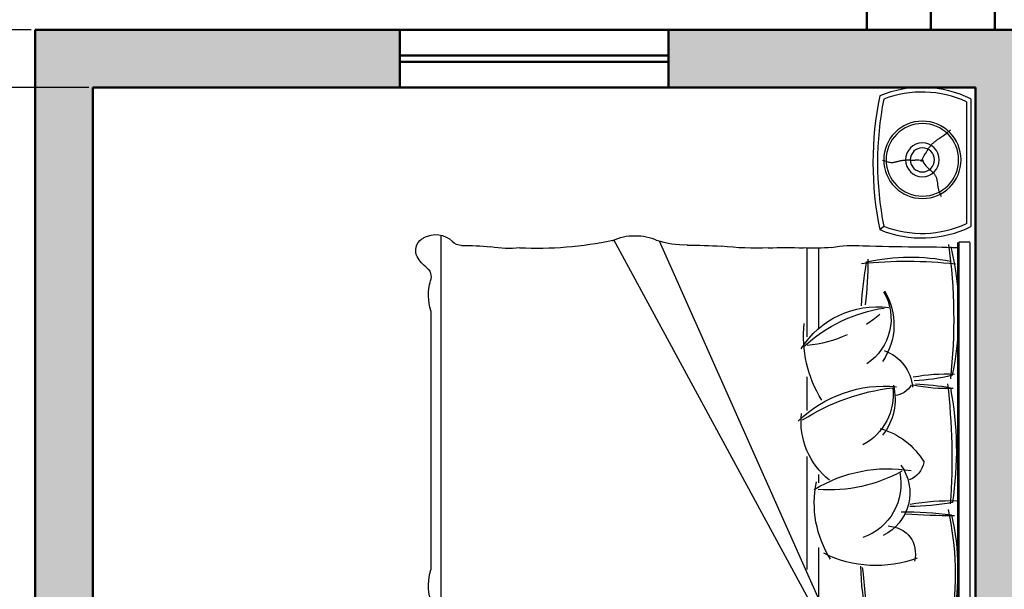
# Model space of a CAD drawing. Units: inches. Extents: x 1986 to 21484, y -1816 to 2016.
# Tile 9 of 85: x 2076 to 2230, y 1765 to 1854. Entities that reach past the tile are written whole.
import ezdxf

# ---------------------------------------------------------------- set-up
doc = ezdxf.new("R2010")
doc.units = ezdxf.units.IN
for name, color, linetype, lineweight in [('A-ANNO-DIMS', 2, 'Continuous', 18), ('A-FURN', 8, 'Continuous', 18), ('A-WALL', 7, 'Continuous', 50), ('A-WALL-PATT', 8, 'Continuous', 13)]:
    doc.layers.add(name, color=color, linetype=linetype, lineweight=lineweight)
doc.layers.add('TEFRİŞ', color=11, linetype='Continuous')
doc.styles.get("Standard").update_dxf_attribs({"font": 'arial.ttf'})
doc.dimstyles.new('ISO-25', dxfattribs={"dimtxt": 8, "dimasz": 2.5, "dimexe": 1.25, "dimexo": 0.625, "dimtad": 1, "dimdec": 1, "dimlunit": 3, "dimtxsty": 'Standard', "dimcen": 2.5, "dimadec": 0, "dimazin": 0, "dimtfac": 1, "dimtdec": 1, "dimtmove": 0, "dimatfit": 3, "dimfxl": 1, "dimarcsym": 0})

# ---------------------------------------------------------------- blocks, each defined once
blk = doc.blocks.new('BED')
at = {"layer": 'TEFRİŞ'}
for p, q in [((2114.88, 1835.66), (2129.12, 1835.66)), ((2177.29, 1835.98), (2177.61, 1835.47)), ((2177.29, 1835.98), (2191.52, 1835.98)), ((2191.2, 1835.47), (2191.52, 1835.98)), ((2115.2, 1835.15), (2128.8, 1835.15)), ((2130.81, 1834.34), (2130.81, 1835.55)), ((2130.91, 1835.55), (2175.56, 1835.55)), ((2175.56, 1835.55), (2175.56, 1834.34)), ((2177.61, 1835.47), (2191.2, 1835.47)), ((2118.49, 1833.2), (2118.34, 1833.38)), ((2118.49, 1833.2), (2118.34, 1833.38)), ((2175.56, 1834.34), (2130.81, 1834.34)), ((2175, 1834.19), (2130.91, 1834.19)), ((2180.9, 1833.52), (2180.75, 1833.7)), ((2180.9, 1833.52), (2180.75, 1833.7)), ((2181.04, 1833.35), (2180.9, 1833.52)), ((2181.04, 1833.35), (2180.9, 1833.52)), ((2118.63, 1833.03), (2118.49, 1833.2)), ((2118.63, 1833.03), (2118.49, 1833.2)), ((2118.75, 1832.88), (2118.63, 1833.03)), ((2118.75, 1832.88), (2118.63, 1833.03)), ((2118.86, 1832.74), (2118.75, 1832.88)), ((2118.86, 1832.74), (2118.75, 1832.88)), ((2118.95, 1832.61), (2118.86, 1832.74)), ((2118.95, 1832.61), (2118.86, 1832.74)), ((2119.04, 1832.48), (2118.95, 1832.61)), ((2119.04, 1832.48), (2118.95, 1832.61)), ((2119.12, 1832.37), (2119.04, 1832.48)), ((2119.12, 1832.37), (2119.04, 1832.48)), ((2119.19, 1832.26), (2119.12, 1832.37)), ((2119.19, 1832.26), (2119.12, 1832.37)), ((2125.6, 1832.25), (2125.68, 1832.3)), ((2125.6, 1832.25), (2125.68, 1832.3)), ((2125.68, 1832.3), (2125.75, 1832.35)), ((2125.68, 1832.3), (2125.75, 1832.35)), ((2181.16, 1833.2), (2181.04, 1833.35)), ((2181.16, 1833.2), (2181.04, 1833.35)), ((2181.26, 1833.06), (2181.16, 1833.2)), ((2181.26, 1833.06), (2181.16, 1833.2)), ((2181.36, 1832.93), (2181.26, 1833.06)), ((2181.36, 1832.93), (2181.26, 1833.06)), ((2181.44, 1832.8), (2181.36, 1832.93)), ((2181.44, 1832.8), (2181.36, 1832.93)), ((2181.52, 1832.69), (2181.44, 1832.8)), ((2181.52, 1832.69), (2181.44, 1832.8)), ((2181.59, 1832.58), (2181.52, 1832.69)), ((2181.59, 1832.58), (2181.52, 1832.69)), ((2181.66, 1832.48), (2181.59, 1832.58)), ((2181.66, 1832.48), (2181.59, 1832.58)), ((2181.73, 1832.38), (2181.66, 1832.48)), ((2181.73, 1832.38), (2181.66, 1832.48)), ((2181.79, 1832.29), (2181.73, 1832.38)), ((2181.79, 1832.29), (2181.73, 1832.38)), ((2181.85, 1832.21), (2181.79, 1832.29)), ((2181.85, 1832.21), (2181.79, 1832.29)), ((2186.9, 1832.26), (2186.97, 1832.27)), ((2186.9, 1832.26), (2186.97, 1832.27)), ((2186.97, 1832.27), (2187.04, 1832.28)), ((2186.97, 1832.27), (2187.04, 1832.28)), ((2187.04, 1832.28), (2187.12, 1832.3)), ((2187.04, 1832.28), (2187.12, 1832.3)), ((2187.12, 1832.3), (2187.2, 1832.31)), ((2187.12, 1832.3), (2187.2, 1832.31)), ((2187.2, 1832.31), (2187.28, 1832.33)), ((2187.2, 1832.31), (2187.28, 1832.33)), ((2187.28, 1832.33), (2187.36, 1832.35)), ((2187.28, 1832.33), (2187.36, 1832.35)), ((2187.36, 1832.35), (2187.45, 1832.37)), ((2187.36, 1832.35), (2187.45, 1832.37)), ((2187.45, 1832.37), (2187.54, 1832.4)), ((2187.45, 1832.37), (2187.54, 1832.4)), ((2187.54, 1832.4), (2187.64, 1832.43)), ((2187.54, 1832.4), (2187.64, 1832.43)), ((2187.64, 1832.43), (2187.74, 1832.46)), ((2187.64, 1832.43), (2187.74, 1832.46)), ((2187.74, 1832.46), (2187.83, 1832.49)), ((2187.74, 1832.46), (2187.83, 1832.49)), ((2187.83, 1832.49), (2187.92, 1832.53)), ((2187.83, 1832.49), (2187.92, 1832.53)), ((2187.92, 1832.53), (2188.01, 1832.57)), ((2187.92, 1832.53), (2188.01, 1832.57)), ((2188.01, 1832.57), (2188.09, 1832.62)), ((2188.01, 1832.57), (2188.09, 1832.62)), ((2188.09, 1832.62), (2188.15, 1832.67)), ((2188.09, 1832.62), (2188.15, 1832.67)), ((2119.26, 1832.16), (2119.19, 1832.26)), ((2119.26, 1832.16), (2119.19, 1832.26)), ((2119.32, 1832.06), (2119.26, 1832.16)), ((2119.32, 1832.06), (2119.26, 1832.16)), ((2119.39, 1831.97), (2119.32, 1832.06)), ((2119.39, 1831.97), (2119.32, 1832.06)), ((2119.45, 1831.89), (2119.39, 1831.97)), ((2119.45, 1831.89), (2119.39, 1831.97)), ((2119.51, 1831.81), (2119.45, 1831.89)), ((2119.51, 1831.81), (2119.45, 1831.89)), ((2119.57, 1831.73), (2119.51, 1831.81)), ((2119.57, 1831.73), (2119.51, 1831.81)), ((2119.63, 1831.65), (2119.57, 1831.73)), ((2119.63, 1831.65), (2119.57, 1831.73)), ((2119.69, 1831.58), (2119.63, 1831.65)), ((2119.69, 1831.58), (2119.63, 1831.65)), ((2119.75, 1831.51), (2119.69, 1831.58)), ((2119.75, 1831.51), (2119.69, 1831.58)), ((2119.81, 1831.44), (2119.75, 1831.51)), ((2119.81, 1831.44), (2119.75, 1831.51)), ((2119.87, 1831.38), (2119.81, 1831.44)), ((2119.87, 1831.38), (2119.81, 1831.44)), ((2119.93, 1831.31), (2119.87, 1831.38)), ((2119.93, 1831.31), (2119.87, 1831.38)), ((2119.99, 1831.25), (2119.93, 1831.31)), ((2119.99, 1831.25), (2119.93, 1831.31)), ((2120.05, 1831.2), (2119.99, 1831.25)), ((2120.05, 1831.2), (2119.99, 1831.25)), ((2120.12, 1831.14), (2120.05, 1831.2)), ((2120.12, 1831.14), (2120.05, 1831.2)), ((2122.8, 1831.09), (2122.87, 1831.18)), ((2122.8, 1831.09), (2122.87, 1831.18)), ((2122.87, 1831.18), (2122.94, 1831.26)), ((2122.87, 1831.18), (2122.94, 1831.26)), ((2122.94, 1831.26), (2123.01, 1831.33)), ((2122.94, 1831.26), (2123.01, 1831.33)), ((2123.01, 1831.33), (2123.08, 1831.4)), ((2123.01, 1831.33), (2123.08, 1831.4)), ((2123.08, 1831.4), (2123.14, 1831.46)), ((2123.08, 1831.4), (2123.14, 1831.46)), ((2123.14, 1831.46), (2123.21, 1831.52)), ((2123.14, 1831.46), (2123.21, 1831.52)), ((2123.21, 1831.52), (2123.27, 1831.58)), ((2123.21, 1831.52), (2123.27, 1831.58)), ((2123.27, 1831.58), (2123.34, 1831.63)), ((2123.27, 1831.58), (2123.34, 1831.63)), ((2123.34, 1831.63), (2123.41, 1831.67)), ((2123.34, 1831.63), (2123.41, 1831.67)), ((2123.41, 1831.67), (2123.48, 1831.71)), ((2123.41, 1831.67), (2123.48, 1831.71)), ((2123.48, 1831.71), (2123.55, 1831.74)), ((2123.48, 1831.71), (2123.55, 1831.74)), ((2123.55, 1831.74), (2123.62, 1831.77)), ((2123.55, 1831.74), (2123.62, 1831.77)), ((2123.62, 1831.77), (2123.69, 1831.8)), ((2123.62, 1831.77), (2123.69, 1831.8)), ((2123.69, 1831.8), (2123.77, 1831.82)), ((2123.69, 1831.8), (2123.77, 1831.82)), ((2123.77, 1831.82), (2123.84, 1831.84)), ((2123.77, 1831.82), (2123.84, 1831.84)), ((2123.84, 1831.84), (2123.91, 1831.86)), ((2123.84, 1831.84), (2123.91, 1831.86)), ((2123.91, 1831.86), (2123.98, 1831.87)), ((2123.91, 1831.86), (2123.98, 1831.87)), ((2123.98, 1831.87), (2124.06, 1831.89)), ((2123.98, 1831.87), (2124.06, 1831.89)), ((2124.06, 1831.89), (2124.13, 1831.9)), ((2124.06, 1831.89), (2124.13, 1831.9)), ((2124.13, 1831.9), (2124.2, 1831.91)), ((2124.13, 1831.9), (2124.2, 1831.91)), ((2124.2, 1831.91), (2124.27, 1831.91)), ((2124.2, 1831.91), (2124.27, 1831.91)), ((2124.27, 1831.91), (2124.35, 1831.92)), ((2124.27, 1831.91), (2124.35, 1831.92)), ((2124.35, 1831.92), (2124.42, 1831.93)), ((2124.35, 1831.92), (2124.42, 1831.93)), ((2124.42, 1831.93), (2124.49, 1831.94)), ((2124.42, 1831.93), (2124.49, 1831.94)), ((2124.49, 1831.94), (2124.56, 1831.95)), ((2124.49, 1831.94), (2124.56, 1831.95)), ((2124.56, 1831.95), (2124.64, 1831.96)), ((2124.56, 1831.95), (2124.64, 1831.96)), ((2124.64, 1831.96), (2124.71, 1831.98)), ((2124.64, 1831.96), (2124.71, 1831.98)), ((2124.71, 1831.98), (2124.79, 1831.99)), ((2124.71, 1831.98), (2124.79, 1831.99)), ((2124.79, 1831.99), (2124.87, 1832.01)), ((2124.79, 1831.99), (2124.87, 1832.01)), ((2124.87, 1832.01), (2124.96, 1832.03)), ((2124.87, 1832.01), (2124.96, 1832.03)), ((2124.96, 1832.03), (2125.05, 1832.05)), ((2124.96, 1832.03), (2125.05, 1832.05)), ((2125.05, 1832.05), (2125.14, 1832.08)), ((2125.05, 1832.05), (2125.14, 1832.08)), ((2125.14, 1832.08), (2125.23, 1832.11)), ((2125.14, 1832.08), (2125.23, 1832.11)), ((2125.23, 1832.11), (2125.33, 1832.14)), ((2125.23, 1832.11), (2125.33, 1832.14)), ((2125.33, 1832.14), (2125.42, 1832.17)), ((2125.33, 1832.14), (2125.42, 1832.17)), ((2125.42, 1832.17), (2125.52, 1832.21)), ((2125.42, 1832.17), (2125.52, 1832.21)), ((2125.52, 1832.21), (2125.6, 1832.25)), ((2125.52, 1832.21), (2125.6, 1832.25)), ((2181.92, 1832.13), (2181.85, 1832.21)), ((2181.92, 1832.13), (2181.85, 1832.21)), ((2181.97, 1832.05), (2181.92, 1832.13)), ((2181.97, 1832.05), (2181.92, 1832.13)), ((2182.03, 1831.97), (2181.97, 1832.05)), ((2182.03, 1831.97), (2181.97, 1832.05)), ((2182.09, 1831.9), (2182.03, 1831.97)), ((2182.09, 1831.9), (2182.03, 1831.97)), ((2182.15, 1831.83), (2182.09, 1831.9)), ((2182.15, 1831.83), (2182.09, 1831.9)), ((2182.21, 1831.76), (2182.15, 1831.83)), ((2182.21, 1831.76), (2182.15, 1831.83)), ((2182.27, 1831.7), (2182.21, 1831.76)), ((2182.27, 1831.7), (2182.21, 1831.76)), ((2182.33, 1831.63), (2182.27, 1831.7)), ((2182.33, 1831.63), (2182.27, 1831.7)), ((2182.4, 1831.57), (2182.33, 1831.63)), ((2182.4, 1831.57), (2182.33, 1831.63)), ((2182.46, 1831.52), (2182.4, 1831.57)), ((2182.46, 1831.52), (2182.4, 1831.57)), ((2182.52, 1831.46), (2182.46, 1831.52)), ((2182.52, 1831.46), (2182.46, 1831.52)), ((2182.59, 1831.41), (2182.52, 1831.46)), ((2182.59, 1831.41), (2182.52, 1831.46)), ((2182.66, 1831.36), (2182.59, 1831.41)), ((2182.66, 1831.36), (2182.59, 1831.41)), ((2182.73, 1831.31), (2182.66, 1831.36)), ((2182.73, 1831.31), (2182.66, 1831.36)), ((2182.8, 1831.26), (2182.73, 1831.31)), ((2182.8, 1831.26), (2182.73, 1831.31)), ((2182.87, 1831.22), (2182.8, 1831.26)), ((2182.87, 1831.22), (2182.8, 1831.26)), ((2182.95, 1831.17), (2182.87, 1831.22)), ((2182.95, 1831.17), (2182.87, 1831.22)), ((2183.03, 1831.12), (2182.95, 1831.17)), ((2183.03, 1831.12), (2182.95, 1831.17)), ((2184.95, 1831.14), (2185.05, 1831.23)), ((2184.95, 1831.14), (2185.05, 1831.23)), ((2185.05, 1831.23), (2185.13, 1831.33)), ((2185.05, 1831.23), (2185.13, 1831.33)), ((2185.13, 1831.33), (2185.21, 1831.41)), ((2185.13, 1831.33), (2185.21, 1831.41)), ((2185.21, 1831.41), (2185.28, 1831.5)), ((2185.21, 1831.41), (2185.28, 1831.5)), ((2185.28, 1831.5), (2185.35, 1831.58)), ((2185.28, 1831.5), (2185.35, 1831.58)), ((2185.35, 1831.58), (2185.42, 1831.65)), ((2185.35, 1831.58), (2185.42, 1831.65)), ((2185.42, 1831.65), (2185.48, 1831.72)), ((2185.42, 1831.65), (2185.48, 1831.72)), ((2185.48, 1831.72), (2185.55, 1831.78)), ((2185.48, 1831.72), (2185.55, 1831.78)), ((2185.55, 1831.78), (2185.61, 1831.84)), ((2185.55, 1831.78), (2185.61, 1831.84)), ((2185.61, 1831.84), (2185.68, 1831.9)), ((2185.61, 1831.84), (2185.68, 1831.9)), ((2185.68, 1831.9), (2185.75, 1831.95)), ((2185.68, 1831.9), (2185.75, 1831.95)), ((2185.75, 1831.95), (2185.82, 1831.99)), ((2185.75, 1831.95), (2185.82, 1831.99)), ((2185.82, 1831.99), (2185.89, 1832.03)), ((2185.82, 1831.99), (2185.89, 1832.03)), ((2185.89, 1832.03), (2185.96, 1832.06)), ((2185.89, 1832.03), (2185.96, 1832.06)), ((2185.96, 1832.06), (2186.03, 1832.09)), ((2185.96, 1832.06), (2186.03, 1832.09)), ((2186.03, 1832.09), (2186.1, 1832.12)), ((2186.03, 1832.09), (2186.1, 1832.12)), ((2186.1, 1832.12), (2186.17, 1832.14)), ((2186.1, 1832.12), (2186.17, 1832.14)), ((2186.17, 1832.14), (2186.24, 1832.16)), ((2186.17, 1832.14), (2186.24, 1832.16)), ((2186.24, 1832.16), (2186.32, 1832.18)), ((2186.24, 1832.16), (2186.32, 1832.18)), ((2186.32, 1832.18), (2186.39, 1832.19)), ((2186.32, 1832.18), (2186.39, 1832.19)), ((2186.39, 1832.19), (2186.46, 1832.21)), ((2186.39, 1832.19), (2186.46, 1832.21)), ((2186.46, 1832.21), (2186.53, 1832.22)), ((2186.46, 1832.21), (2186.53, 1832.22)), ((2186.53, 1832.22), (2186.61, 1832.23)), ((2186.53, 1832.22), (2186.61, 1832.23)), ((2186.61, 1832.23), (2186.68, 1832.23)), ((2186.61, 1832.23), (2186.68, 1832.23)), ((2186.68, 1832.23), (2186.75, 1832.24)), ((2186.68, 1832.23), (2186.75, 1832.24)), ((2186.75, 1832.24), (2186.82, 1832.25)), ((2186.75, 1832.24), (2186.82, 1832.25)), ((2186.82, 1832.25), (2186.9, 1832.26)), ((2186.82, 1832.25), (2186.9, 1832.26)), ((2120.18, 1831.09), (2120.12, 1831.14)), ((2120.18, 1831.09), (2120.12, 1831.14)), ((2120.25, 1831.04), (2120.18, 1831.09)), ((2120.25, 1831.04), (2120.18, 1831.09)), ((2120.32, 1830.99), (2120.25, 1831.04)), ((2120.32, 1830.99), (2120.25, 1831.04)), ((2120.39, 1830.94), (2120.32, 1830.99)), ((2120.39, 1830.94), (2120.32, 1830.99)), ((2120.47, 1830.9), (2120.39, 1830.94)), ((2120.47, 1830.9), (2120.39, 1830.94)), ((2120.54, 1830.85), (2120.47, 1830.9)), ((2120.54, 1830.85), (2120.47, 1830.9)), ((2120.62, 1830.8), (2120.54, 1830.85)), ((2120.62, 1830.8), (2120.54, 1830.85)), ((2120.7, 1830.75), (2120.62, 1830.8)), ((2120.7, 1830.75), (2120.62, 1830.8)), ((2120.79, 1830.7), (2120.7, 1830.75)), ((2120.79, 1830.7), (2120.7, 1830.75)), ((2120.88, 1830.65), (2120.79, 1830.7)), ((2120.88, 1830.65), (2120.79, 1830.7)), ((2120.98, 1830.59), (2120.88, 1830.65)), ((2120.98, 1830.59), (2120.88, 1830.65)), ((2121.09, 1830.52), (2120.98, 1830.59)), ((2121.09, 1830.52), (2120.98, 1830.59)), ((2121.21, 1830.45), (2121.09, 1830.52)), ((2121.21, 1830.45), (2121.09, 1830.52)), ((2121.34, 1830.38), (2121.21, 1830.45)), ((2121.34, 1830.38), (2121.21, 1830.45)), ((2121.49, 1830.29), (2121.34, 1830.38)), ((2121.49, 1830.29), (2121.34, 1830.38)), ((2121.66, 1830.21), (2121.49, 1830.29)), ((2121.66, 1830.21), (2121.49, 1830.29)), ((2121.66, 1830.18), (2121.87, 1830.29)), ((2121.66, 1830.18), (2121.87, 1830.29)), ((2121.85, 1830.11), (2121.66, 1830.21)), ((2121.85, 1830.11), (2121.66, 1830.21)), ((2121.76, 1830.38), (2121.74, 1830.17)), ((2121.76, 1830.38), (2121.74, 1830.17)), ((2121.74, 1830.17), (2121.74, 1829.99)), ((2121.74, 1830.17), (2121.74, 1829.99)), ((2121.87, 1830.29), (2122.04, 1830.4)), ((2121.87, 1830.29), (2122.04, 1830.4)), ((2122.04, 1830.4), (2122.2, 1830.51)), ((2122.04, 1830.4), (2122.2, 1830.51)), ((2122.2, 1830.51), (2122.33, 1830.61)), ((2122.2, 1830.51), (2122.33, 1830.61)), ((2122.33, 1830.61), (2122.45, 1830.72)), ((2122.33, 1830.61), (2122.45, 1830.72)), ((2122.45, 1830.72), (2122.55, 1830.82)), ((2122.45, 1830.72), (2122.55, 1830.82)), ((2122.55, 1830.82), (2122.64, 1830.91)), ((2122.55, 1830.82), (2122.64, 1830.91)), ((2122.64, 1830.91), (2122.72, 1831.01)), ((2122.64, 1830.91), (2122.72, 1831.01)), ((2122.72, 1831.01), (2122.8, 1831.09)), ((2122.72, 1831.01), (2122.8, 1831.09)), ((2183.11, 1831.07), (2183.03, 1831.12)), ((2183.11, 1831.07), (2183.03, 1831.12)), ((2183.2, 1831.02), (2183.11, 1831.07)), ((2183.2, 1831.02), (2183.11, 1831.07)), ((2183.29, 1830.97), (2183.2, 1831.02)), ((2183.29, 1830.97), (2183.2, 1831.02)), ((2183.39, 1830.91), (2183.29, 1830.97)), ((2183.39, 1830.91), (2183.29, 1830.97)), ((2183.49, 1830.84), (2183.39, 1830.91)), ((2183.49, 1830.84), (2183.39, 1830.91)), ((2183.61, 1830.77), (2183.49, 1830.84)), ((2183.61, 1830.77), (2183.49, 1830.84)), ((2183.75, 1830.7), (2183.61, 1830.77)), ((2183.75, 1830.7), (2183.61, 1830.77)), ((2183.9, 1830.61), (2183.75, 1830.7)), ((2183.9, 1830.61), (2183.75, 1830.7)), ((2184.06, 1830.53), (2183.9, 1830.61)), ((2184.06, 1830.53), (2183.9, 1830.61)), ((2184.25, 1830.43), (2184.06, 1830.53)), ((2184.25, 1830.43), (2184.06, 1830.53)), ((2184.07, 1830.5), (2184.27, 1830.61)), ((2184.07, 1830.5), (2184.27, 1830.61)), ((2184.15, 1830.49), (2184.14, 1830.31)), ((2184.15, 1830.49), (2184.14, 1830.31)), ((2184.14, 1830.31), (2184.14, 1830.15)), ((2184.14, 1830.31), (2184.14, 1830.15)), ((2184.14, 1830.15), (2184.14, 1830.01)), ((2184.14, 1830.15), (2184.14, 1830.01)), ((2184.17, 1830.7), (2184.15, 1830.49)), ((2184.17, 1830.7), (2184.15, 1830.49)), ((2184.27, 1830.61), (2184.45, 1830.72)), ((2184.27, 1830.61), (2184.45, 1830.72)), ((2184.45, 1830.72), (2184.6, 1830.83)), ((2184.45, 1830.72), (2184.6, 1830.83)), ((2184.6, 1830.83), (2184.74, 1830.93)), ((2184.6, 1830.83), (2184.74, 1830.93)), ((2184.74, 1830.93), (2184.85, 1831.04)), ((2184.74, 1830.93), (2184.85, 1831.04)), ((2184.85, 1831.04), (2184.95, 1831.14)), ((2184.85, 1831.04), (2184.95, 1831.14)), ((2121.74, 1829.99), (2121.73, 1829.83)), ((2121.74, 1829.99), (2121.73, 1829.83)), ((2121.73, 1829.83), (2121.73, 1829.69)), ((2121.73, 1829.83), (2121.73, 1829.69)), ((2121.73, 1829.69), (2121.73, 1829.57)), ((2121.73, 1829.69), (2121.73, 1829.57)), ((2121.73, 1829.57), (2121.73, 1829.45)), ((2121.73, 1829.57), (2121.73, 1829.45)), ((2121.73, 1829.45), (2121.74, 1829.35)), ((2121.73, 1829.45), (2121.74, 1829.35)), ((2121.74, 1829.35), (2121.74, 1829.25)), ((2121.74, 1829.35), (2121.74, 1829.25)), ((2121.74, 1829.25), (2121.74, 1829.16)), ((2121.74, 1829.25), (2121.74, 1829.16)), ((2121.74, 1829.16), (2121.74, 1829.06)), ((2121.74, 1829.16), (2121.74, 1829.06)), ((2121.74, 1829.06), (2121.74, 1828.97)), ((2121.74, 1829.06), (2121.74, 1828.97)), ((2121.74, 1828.97), (2121.74, 1828.89)), ((2121.74, 1828.97), (2121.74, 1828.89)), ((2184.14, 1829.04), (2184.13, 1828.96)), ((2184.14, 1829.04), (2184.13, 1828.96)), ((2184.14, 1830.01), (2184.14, 1829.89)), ((2184.14, 1830.01), (2184.14, 1829.89)), ((2184.14, 1829.89), (2184.14, 1829.77)), ((2184.14, 1829.89), (2184.14, 1829.77)), ((2184.14, 1829.77), (2184.14, 1829.67)), ((2184.14, 1829.77), (2184.14, 1829.67)), ((2184.14, 1829.67), (2184.15, 1829.57)), ((2184.14, 1829.67), (2184.15, 1829.57)), ((2184.15, 1829.38), (2184.14, 1829.29)), ((2184.15, 1829.38), (2184.14, 1829.29)), ((2184.14, 1829.29), (2184.14, 1829.21)), ((2184.14, 1829.29), (2184.14, 1829.21)), ((2184.14, 1829.21), (2184.14, 1829.12)), ((2184.14, 1829.21), (2184.14, 1829.12)), ((2184.14, 1829.12), (2184.14, 1829.04)), ((2184.14, 1829.12), (2184.14, 1829.04)), ((2184.15, 1829.57), (2184.15, 1829.48)), ((2184.15, 1829.57), (2184.15, 1829.48)), ((2184.15, 1829.48), (2184.15, 1829.38)), ((2184.15, 1829.48), (2184.15, 1829.38)), ((2121.74, 1828.89), (2121.73, 1828.8)), ((2121.74, 1828.89), (2121.73, 1828.8)), ((2121.73, 1828.8), (2121.73, 1828.72)), ((2121.73, 1828.8), (2121.73, 1828.72)), ((2121.73, 1828.72), (2121.73, 1828.64)), ((2121.73, 1828.72), (2121.73, 1828.64)), ((2121.73, 1828.64), (2121.73, 1828.56)), ((2121.73, 1828.64), (2121.73, 1828.56)), ((2121.73, 1828.56), (2121.73, 1828.48)), ((2121.73, 1828.56), (2121.73, 1828.48)), ((2121.73, 1828.48), (2121.73, 1828.4)), ((2121.73, 1828.48), (2121.73, 1828.4)), ((2121.73, 1828.4), (2121.73, 1828.33)), ((2121.73, 1828.4), (2121.73, 1828.33)), ((2121.73, 1828.33), (2121.74, 1828.25)), ((2121.73, 1828.33), (2121.74, 1828.25)), ((2121.74, 1828.25), (2121.75, 1828.18)), ((2121.74, 1828.25), (2121.75, 1828.18)), ((2121.75, 1828.18), (2121.75, 1828.1)), ((2121.75, 1828.18), (2121.75, 1828.1)), ((2121.75, 1828.1), (2121.76, 1828.03)), ((2121.75, 1828.1), (2121.76, 1828.03)), ((2121.76, 1828.03), (2121.78, 1827.95)), ((2121.76, 1828.03), (2121.78, 1827.95)), ((2121.78, 1827.95), (2121.79, 1827.88)), ((2121.78, 1827.95), (2121.79, 1827.88)), ((2121.79, 1827.88), (2121.8, 1827.8)), ((2121.79, 1827.88), (2121.8, 1827.8)), ((2184.13, 1828.96), (2184.13, 1828.88)), ((2184.13, 1828.96), (2184.13, 1828.88)), ((2184.13, 1828.88), (2184.13, 1828.8)), ((2184.13, 1828.88), (2184.13, 1828.8)), ((2184.13, 1828.8), (2184.14, 1828.72)), ((2184.13, 1828.8), (2184.14, 1828.72)), ((2184.14, 1828.72), (2184.14, 1828.65)), ((2184.14, 1828.72), (2184.14, 1828.65)), ((2184.14, 1828.65), (2184.15, 1828.57)), ((2184.14, 1828.65), (2184.15, 1828.57)), ((2184.15, 1828.57), (2184.15, 1828.5)), ((2184.15, 1828.57), (2184.15, 1828.5)), ((2184.15, 1828.5), (2184.16, 1828.42)), ((2184.15, 1828.5), (2184.16, 1828.42)), ((2184.16, 1828.42), (2184.17, 1828.35)), ((2184.16, 1828.42), (2184.17, 1828.35)), ((2184.17, 1828.35), (2184.18, 1828.27)), ((2184.17, 1828.35), (2184.18, 1828.27)), ((2184.18, 1828.27), (2184.19, 1828.2)), ((2184.18, 1828.27), (2184.19, 1828.2)), ((2184.19, 1828.2), (2184.21, 1828.12)), ((2184.19, 1828.2), (2184.21, 1828.12)), ((2184.21, 1828.12), (2184.22, 1828.04)), ((2184.21, 1828.12), (2184.22, 1828.04)), ((2184.22, 1828.04), (2184.24, 1827.97)), ((2184.22, 1828.04), (2184.24, 1827.97)), ((2184.24, 1827.97), (2184.26, 1827.89)), ((2184.24, 1827.97), (2184.26, 1827.89)), ((2184.26, 1827.89), (2184.28, 1827.81)), ((2184.26, 1827.89), (2184.28, 1827.81)), ((2121.8, 1827.8), (2121.82, 1827.72)), ((2121.8, 1827.8), (2121.82, 1827.72)), ((2121.82, 1827.72), (2121.84, 1827.65)), ((2121.82, 1827.72), (2121.84, 1827.65)), ((2121.84, 1827.65), (2121.85, 1827.57)), ((2121.84, 1827.65), (2121.85, 1827.57)), ((2121.85, 1827.57), (2121.87, 1827.49)), ((2121.85, 1827.57), (2121.87, 1827.49)), ((2121.87, 1827.49), (2121.89, 1827.41)), ((2121.87, 1827.49), (2121.89, 1827.41)), ((2121.89, 1827.41), (2121.91, 1827.33)), ((2121.89, 1827.41), (2121.91, 1827.33)), ((2121.91, 1827.33), (2121.93, 1827.26)), ((2121.91, 1827.33), (2121.93, 1827.26)), ((2121.93, 1827.26), (2121.95, 1827.18)), ((2121.93, 1827.26), (2121.95, 1827.18)), ((2121.95, 1827.18), (2121.97, 1827.09)), ((2121.95, 1827.18), (2121.97, 1827.09)), ((2121.97, 1827.09), (2121.99, 1827.01)), ((2121.97, 1827.09), (2121.99, 1827.01)), ((2121.99, 1827.01), (2122, 1826.93)), ((2121.99, 1827.01), (2122, 1826.93)), ((2122, 1826.93), (2122.01, 1826.84)), ((2122, 1826.93), (2122.01, 1826.84)), ((2122.01, 1826.84), (2122, 1826.74)), ((2122.01, 1826.84), (2122, 1826.74)), ((2184.28, 1827.81), (2184.3, 1827.73)), ((2184.28, 1827.81), (2184.3, 1827.73)), ((2184.3, 1827.73), (2184.32, 1827.65)), ((2184.3, 1827.73), (2184.32, 1827.65)), ((2184.32, 1827.65), (2184.34, 1827.58)), ((2184.32, 1827.65), (2184.34, 1827.58)), ((2184.34, 1827.58), (2184.36, 1827.5)), ((2184.34, 1827.58), (2184.36, 1827.5)), ((2184.38, 1826.86), (2184.35, 1826.74)), ((2184.38, 1826.86), (2184.35, 1826.74)), ((2184.36, 1827.5), (2184.38, 1827.41)), ((2184.36, 1827.5), (2184.38, 1827.41)), ((2184.38, 1827.41), (2184.4, 1827.33)), ((2184.38, 1827.41), (2184.4, 1827.33)), ((2184.4, 1826.96), (2184.38, 1826.86)), ((2184.4, 1826.96), (2184.38, 1826.86)), ((2184.4, 1827.33), (2184.41, 1827.25)), ((2184.4, 1827.33), (2184.41, 1827.25)), ((2184.41, 1827.06), (2184.4, 1826.96)), ((2184.41, 1827.06), (2184.4, 1826.96)), ((2184.41, 1827.25), (2184.41, 1827.16)), ((2184.41, 1827.25), (2184.41, 1827.16)), ((2184.41, 1827.16), (2184.41, 1827.06)), ((2184.41, 1827.16), (2184.41, 1827.06)), ((2121.78, 1825.93), (2121.74, 1825.8)), ((2121.78, 1825.93), (2121.74, 1825.8)), ((2121.83, 1826.06), (2121.78, 1825.93)), ((2121.83, 1826.06), (2121.78, 1825.93)), ((2121.87, 1826.19), (2121.83, 1826.06)), ((2121.87, 1826.19), (2121.83, 1826.06)), ((2121.91, 1826.31), (2121.87, 1826.19)), ((2121.91, 1826.31), (2121.87, 1826.19)), ((2121.95, 1826.42), (2121.91, 1826.31)), ((2121.95, 1826.42), (2121.91, 1826.31)), ((2121.97, 1826.54), (2121.95, 1826.42)), ((2121.97, 1826.54), (2121.95, 1826.42)), ((2121.99, 1826.64), (2121.97, 1826.54)), ((2121.99, 1826.64), (2121.97, 1826.54)), ((2122, 1826.74), (2121.99, 1826.64)), ((2122, 1826.74), (2121.99, 1826.64)), ((2129.46, 1825.49), (2129.09, 1825.93)), ((2176.94, 1825.81), (2177.31, 1826.25)), ((2184.19, 1826.25), (2184.14, 1826.12)), ((2184.19, 1826.25), (2184.14, 1826.12)), ((2184.23, 1826.38), (2184.19, 1826.25)), ((2184.23, 1826.38), (2184.19, 1826.25)), ((2184.28, 1826.51), (2184.23, 1826.38)), ((2184.28, 1826.51), (2184.23, 1826.38)), ((2184.32, 1826.63), (2184.28, 1826.51)), ((2184.32, 1826.63), (2184.28, 1826.51)), ((2184.35, 1826.74), (2184.32, 1826.63)), ((2184.35, 1826.74), (2184.32, 1826.63)), ((2191.87, 1825.81), (2191.5, 1826.25)), ((2174.77, 1820.53), (2130.76, 1800.91)), ((2174.77, 1819.77), (2130.6, 1795.83)), ((2140.43, 1818.69), (2131.53, 1818.69)), ((2157.71, 1818.69), (2156.77, 1818.69)), ((2170.41, 1818.69), (2164.92, 1818.69)), ((2141.43, 1817.4), (2131.53, 1817.4)), ((2149.62, 1817.4), (2145.88, 1817.4)), ((2167.36, 1817.4), (2154.77, 1817.4)), ((2175, 1776.57), (2130.11, 1776.57)), ((2138.52, 1775.41), (2167.39, 1775.41))]:
    blk.add_line(p, q, dxfattribs=at)
for centre, radius, start, end in [((2126, 1830.19), 12.39, 153.8162, 202.314), ((2118, 1830.19), 12.39, 337.686, 26.1838), ((2188.4, 1830.51), 12.39, 153.8162, 202.314), ((2180.41, 1830.51), 12.39, 337.686, 26.1838), ((2126, 1830.19), 11.88, 155.3335, 201.0157), ((2118, 1830.19), 11.88, 338.9843, 24.6665), ((2188.4, 1830.51), 11.88, 155.3335, 201.0157), ((2180.41, 1830.51), 11.88, 338.9843, 24.6665), ((2122, 1861.35), 36.12, 258.6773, 281.3227), ((2184.41, 1861.67), 36.63, 258.2443, 281.7557), ((2184.41, 1861.67), 36.12, 258.6773, 281.3227), ((2122, 1861.35), 36.63, 258.2443, 281.7557)]:
    blk.add_arc(centre, radius, start, end, dxfattribs=at)
at = {"layer": 'TEFRİŞ', "extrusion": (0, 0, -1)}
for centre, major_axis, ratio, start_param, end_param in [((2121.68, 1830.24), (-3.05, -3.05), 1, 3.926991, 10.210176), ((2121.68, 1830.24), (2.86, -2.86), 1, 5.497787, 11.780972), ((2121.68, 1830.24), (2.86, -2.86), 1, 5.497787, 11.780972), ((2138.85, 1803.05), (-22.1, 22.1), 1, 0.544604, 1.006234), ((2184.09, 1830.56), (-3.05, -3.05), 1, 3.926991, 10.210176), ((2184.09, 1830.56), (2.86, -2.86), 1, 5.497787, 11.780972), ((2184.09, 1830.56), (2.86, -2.86), 1, 5.497787, 11.780972), ((2139.43, 1773.84), (-42.35, 42.35), 1, 0.646251, 0.896949), ((2206.14, 1830.73), (-52.86, -52.86), 1, 0.767743, 0.83177), ((2154.7, 1828.89), (-15.68, 15.68), 1, -1.00675, -0.580436), ((2181.61, 1828.44), (-34.39, 34.39), 1, -0.888486, -0.672463), ((2164.51, 1832.79), (-13.41, 13.41), 1, -0.974476, -0.730892), ((2127.6, 1828.81), (-13.23, 13.23), 1, 2.100388, 2.328052), ((2155, 1761.9), (-50.65, -50.65), 1, 2.239512, 2.426533), ((2172.01, 1828.66), (-17.93, 17.93), 1, -0.753394, -0.598744), ((2128.44, 1832.96), (-13.26, -13.26), 1, 3.889049, 4.127298), ((2154.12, 1796.61), (-26.46, 26.46), 1, 0.596409, 0.940188), ((2183.72, 1833.22), (-17, 17), 1, -0.967105, -0.749712), ((2134, 1828.8), (-18.62, 18.62), 1, 2.173461, 2.355043), ((2168.35, 1789.27), (-1.33, 44.62), 0.875277, -0.163954, 0.163954), ((2199.2, 1828.45), (-27.06, -27.06), 1, 0.770625, 0.917228), ((2087.32, 1833.96), (-52.37, 52.37), 1, 2.358049, 2.431787), ((2167.6, 1797.72), (-0.51, 36.47), 0.865194, -0.185965, 0.185965), ((2164.15, 1828.7), (-6.99, 6.99), 1, 1.789136, 2.946702), ((2156.76, 1828.98), (-11.9, -11.9), 1, 3.646453, 4.226155), ((2099.77, 1830.73), (-52.86, 52.86), 1, 2.311571, 2.373849), ((2184.09, 1830.56), (1.33, -1.33), 1, 5.497787, 11.780972), ((2184.09, 1830.56), (1.33, -1.33), 1, 5.497787, 11.780972), ((2121.68, 1830.24), (1.33, -1.33), 1, 5.497787, 11.780972), ((2121.68, 1830.24), (1.33, -1.33), 1, 5.497787, 11.780972), ((2121.68, 1830.24), (0.952, -0.952), 1, 5.497787, 11.780972), ((2121.68, 1830.24), (0.952, -0.952), 1, 5.497787, 11.780972), ((2184.09, 1830.56), (0.952, -0.952), 1, 5.497787, 11.780972), ((2184.09, 1830.56), (0.952, -0.952), 1, 5.497787, 11.780972), ((2159.55, 1823.33), (-5.81, 5.81), 1, -0.516587, 0.256776), ((2154.84, 1827.75), (-1.93, 1.93), 1, 0.997904, 1.977819), ((2675.38, 1815.09), (-384.79, -384.79), 1, 0.80103, 0.811711), ((2147.44, 1824.41), (-3.36, -3.36), 1, 1.11934, 2.270556), ((2145.66, 1827.01), (-1.62, 1.62), 1, 1.310976, 2.284591), ((2172, 1826.44), (-11.23, 11.23), 1, -1.332486, -0.624868), ((2158.82, 1823.55), (-3.74, -3.74), 1, 1.730792, 3.47045), ((2166.67, 1824.96), (-2.93, 3.91), 0.760601, -0.723751, 0.723751), ((2153.88, 1825.05), (-9.22, 9.22), 1, 1.994956, 2.818753), ((1630.53, 1815.09), (-384.79, 384.79), 1, 2.329881, 2.340562), ((2141.71, 1819.83), (-11.86, 11.86), 1, 1.850844, 2.42862), ((2157.83, 1821.53), (-4.47, 4.47), 1, 0.576679, 2.021689), ((2140.05, 1819.86), (-5.1, 5.1), 1, 0.238357, 1.390139), ((2139.42, 1820.79), (-4.21, -4.21), 1, 1.82161, 3.349145), ((2160.6, 1825.98), (-9.68, -9.68), 1, 0.009196, 0.886853), ((2148.35, 1820.65), (-4.63, -4.63), 1, 2.117602, 3.020837), ((2147.86, 1820.64), (-4.48, 4.48), 1, 0.665914, 1.867503), ((2170.68, 1829.67), (-16.79, 16.79), 1, -1.354718, -0.902276), ((2148.15, 1825.25), (-7.14, -7.14), 1, 6.061986, 7.190757), ((2154.93, 1828.48), (-11.96, 11.96), 1, -1.530302, -0.934407), ((2127.37, 1815.76), (-10.68, 10.68), 1, 1.657204, 1.779381), ((2146.08, 1822.57), (-10.5, 10.5), 1, -0.951783, -0.716225), ((2132.43, 1774.09), (-35.41, -35.41), 1, 2.362911, 2.464592), ((2140.17, 1862.96), (-27.99, 27.99), 1, 3.983025, 4.107469), ((2165.73, 1860.69), (-26.41, -26.41), 1, 5.306413, 5.463767), ((2199.62, 1529.47), (-209.2, 209.2), 1, 0.675361, 0.697001), ((2159.82, 1822.57), (-10.5, -10.5), 1, 3.857817, 4.093375), ((2127.37, 1815.76), (-10.68, 10.68), 1, 1.94252, 2.248924), ((2111.06, 1818.12), (-14.48, 14.48), 1, 2.258605, 2.412359), ((2150.79, 1825.18), (-6, 6), 1, 3.032122, 4.026148), ((2159.02, 1834.9), (-3.04, 16.53), 0.830169, 2.822117, 3.461068), ((2194.85, 1818.12), (-14.48, 14.48), 1, -0.841563, -0.687809), ((2141.33, 1830.48), (-9.55, -9.55), 1, 4.941413, 5.601673), ((2169.92, 1815.01), (-27.2, -27.2), 1, 0.734393, 0.836404), ((2135.98, 1815.01), (-27.2, -27.2), 1, 3.875985, 3.977996), ((2098.24, 1811.68), (-23.54, -23.54), 1, 3.885834, 4.043401), ((2207.66, 1811.68), (-23.54, -23.54), 1, 0.668988, 0.826555), ((2189.03, 1803.74), (-40.91, -40.91), 1, 0.789771, 0.855756), ((2116.87, 1803.74), (-40.91, 40.91), 1, 2.285836, 2.351822), ((2122.14, 1803.63), (-6.39, -6.39), 1, 3.886359, 4.265474), ((2222.76, 1798.77), (-34.16, -34.16), 1, 0.743488, 0.893627), ((2135.02, 1798.41), (-3.45, 3.45), 1, -0.831635, -0.314979), ((2135.48, 1798), (-3.77, -3.77), 1, 0.329385, 0.820948), ((2148.06, 1790.38), (-0.75, 67.37), 0.394952, 1.480524, 1.661068), ((2127.76, 1790.23), (-1, 12.37), 0.296708, 1.141067, 2.000525), ((2118.49, 1784.2), (-9.24, -9.24), 1, 3.839645, 4.088086), ((2182.27, 1782.99), (-5.52, -5.52), 1, 0.671703, 0.993321), ((2162.12, 1778.86), (-21.85, 21.85), 1, -0.78611, -0.680117), ((2143.78, 1778.86), (-21.85, 21.85), 1, 2.250913, 2.356906), ((2129.83, 1778.8), (-0.986, 0.986), 1, 2.330985, 3.163296), ((2176.08, 1778.8), (-0.986, 0.986), 1, 4.690686, 5.522997), ((2132.72, 1775.92), (-1.91, -1.91), 1, 0.284117, 1.557111), ((2173.18, 1775.92), (-1.91, -1.91), 1, 3.155278, 4.428271), ((2134.73, 1774.06), (-0.964, -0.964), 1, 1.381176, 2.701227), ((2136.75, 1781.14), (-4.24, 4.24), 1, 3.62713, 4.188813), ((2169.16, 1781.14), (-4.24, 4.24), 1, 3.665169, 4.226852), ((2171.17, 1774.06), (-0.964, -0.964), 1, 2.011162, 3.331212), ((2131.79, 1775.28), (-1.11, 1.11), 1, 3.629269, 5.067473), ((2130.83, 1777), (-2.49, -2.49), 1, 4.590984, 5.084038), ((2175.07, 1777), (-2.49, 2.49), 1, 4.34074, 4.833793), ((2174.12, 1775.28), (-1.11, 1.11), 1, 2.786508, 4.224712)]:
    blk.add_ellipse(centre, major_axis=major_axis, ratio=ratio, start_param=start_param, end_param=end_param, dxfattribs=at)
blk = doc.blocks.new('*D135')
at = {"layer": 'A-ANNO-DIMS', "color": 0, "lineweight": -2, "transparency": 16777216}
for p, q in [((2077.69, 1852.75), (1994.81, 1852.75)), ((1996.06, 1850.25), (1996.06, 1846.25)), ((2086.69, 1843.75), (1994.81, 1843.75)), ((1996.06, 1843.75), (1996.06, 1818.74))]:
    blk.add_line(p, q, dxfattribs=at)
at = {"layer": 'A-ANNO-DIMS', "color": 0, "transparency": 16777216}
for points in [[(1995.65, 1850.25), (1996.48, 1850.25), (1996.06, 1852.75)], [(1995.65, 1846.25), (1996.48, 1846.25), (1996.06, 1843.75)]]:
    blk.add_solid(points, dxfattribs=at)
at = {"layer": 'Defpoints', "color": 0, "transparency": 16777216}
for p in [(2078.31, 1852.75), (1996.06, 1843.75), (2087.31, 1843.75)]:
    blk.add_point(p, dxfattribs=at)
at = {"layer": 'A-ANNO-DIMS', "color": 0, "transparency": 16777216, "insert": (1991.35, 1829.99), "char_height": 8, "attachment_point": 5, "rotation": 90}
blk.add_mtext('0\'-9"', dxfattribs=at)

msp = doc.modelspace()

# ---------------------------------------------------------------- hatches: boundary and pattern name
at = {"layer": 'A-WALL-PATT'}
h = msp.add_hatch(color=256, dxfattribs=at)
h.dxf.hatch_style = 1
h.paths.add_polyline_path([(2087.31, 1843.75), (2135.31, 1843.75), (2135.31, 1852.75), (2078.31, 1852.75), (2078.31, 1753.75), (2087.31, 1753.75)])
h.paths.add_polyline_path([(2231.31, 1852.75), (2177.31, 1852.75), (2177.31, 1843.75), (2225.31, 1843.75), (2225.31, 1627.75), (2231.31, 1627.75), (2231.31, 1633.35), (2231.31, 1676.45), (2231.31, 1678.13)])
h.paths.add_polyline_path([(2384.31, 1852.75), (2261.31, 1852.75), (2261.31, 1843.75), (2375.31, 1843.75), (2375.31, 1795.75), (2279.31, 1795.75), (2279.31, 1813.75), (2273.31, 1813.75), (2273.31, 1789.75), (2375.31, 1789.75), (2375.31, 1741.75), (2384.31, 1741.75)])
h.paths.add_polyline_path([(2384.31, 1705.75), (2375.31, 1705.75), (2375.31, 1600.75), (2384.31, 1600.75)])
h.paths.add_polyline_path([(2384.31, 1564.75), (2375.31, 1564.75), (2375.31, 1537.75), (2293.31, 1537.75), (2293.31, 1531.75), (2375.31, 1531.75), (2384.31, 1531.75)])
h.paths.add_polyline_path([(2087.31, 1711.75), (2078.31, 1711.75), (2078.31, 1669.75), (2087.31, 1669.75), (2087.31, 1681.75), (2177.31, 1681.75), (2177.31, 1663.75), (2183.31, 1663.75), (2183.31, 1681.75), (2189.31, 1681.75), (2189.31, 1687.75), (2087.31, 1687.75)])
h.paths.add_polyline_path([(2087.31, 1627.75), (2183.31, 1627.75), (2183.31, 1633.75), (2153.31, 1633.75), (2087.31, 1633.75), (2087.31, 1645.75), (2078.31, 1645.75), (2078.31, 1441.75), (2087.31, 1441.75)])
h.paths.add_polyline_path([(2087.31, 1399.75), (2078.31, 1399.75), (2078.31, 1276.75), (2087.31, 1276.75)])
h.paths.add_polyline_path([(2151.81, 1387.75), (2135.31, 1387.75), (2135.31, 1378.75), (2151.81, 1378.75)])
h.paths.add_polyline_path([(2219.31, 1387.75), (2193.81, 1387.75), (2193.81, 1378.75), (2210.31, 1378.75), (2210.31, 1189.75), (2219.31, 1189.75)])
h.paths.add_polyline_path([(2384.31, 1387.75), (2375.31, 1387.75), (2255.31, 1387.75), (2255.31, 1381.75), (2375.31, 1381.75), (2375.31, 1363.75), (2384.31, 1363.75)])
h.paths.add_polyline_path([(2384.31, 1339.75), (2375.31, 1339.75), (2375.31, 1321.75), (2279.31, 1321.75), (2279.31, 1351.75), (2273.31, 1351.75), (2273.31, 1315.75), (2375.31, 1315.75), (2375.31, 1303.75), (2384.31, 1303.75)])
h.paths.add_polyline_path([(2225.31, 1123.75), (2219.31, 1123.75), (2219.31, 1147.75), (2210.31, 1147.75), (2210.31, 1114.75), (2225.31, 1114.75)])
h.paths.add_polyline_path([(2384.31, 1147.75), (2375.31, 1147.75), (2375.31, 1123.75), (2267.31, 1123.75), (2267.31, 1114.75), (2384.31, 1114.75)])
h.paths.add_polyline_path([(2384.31, 1261.75), (2375.31, 1261.75), (2375.31, 1189.75), (2384.31, 1189.75)])
h.paths.add_polyline_path([(2384.31, 1441.75), (2375.31, 1441.75), (2375.31, 1423.75), (2384.31, 1423.75)])
h.paths.add_polyline_path([(2384.31, 1495.75), (2375.31, 1495.75), (2375.31, 1477.75), (2384.31, 1477.75)])

# ---------------------------------------------------------------- linework, layer by layer
at = {"layer": 'A-WALL'}
for p, q in [((2208.31, 1900.75), (2208.31, 1852.75)), ((2218.31, 1900.75), (2218.31, 1852.75)), ((2228.31, 1900.75), (2228.31, 1852.75)), ((2078.31, 1852.75), (2231.31, 1852.75)), ((2078.31, 1276.75), (2078.31, 1852.75)), ((2135.31, 1843.75), (2135.31, 1852.75)), ((2177.31, 1843.75), (2177.31, 1852.75)), ((2135.31, 1848.75), (2177.31, 1848.75)), ((2135.31, 1847.75), (2177.31, 1847.75)), ((2087.31, 1843.75), (2225.31, 1843.75)), ((2087.31, 1687.75), (2087.31, 1843.75)), ((2225.31, 1627.75), (2225.31, 1843.75))]:
    msp.add_line(p, q, dxfattribs=at)

# ---------------------------------------------------------------- block references
at = {"layer": 'A-FURN', "xscale": 1.401381342801572, "yscale": 1.401381342801572, "zscale": 1.401381342801572, "rotation": 270}
msp.add_blockref('BED', (-347.86, 4805.72), dxfattribs=at)

# ---------------------------------------------------------------- dimensions: what is measured, and where the dimension line sits
at = {"layer": 'A-ANNO-DIMS'}
dim = msp.add_linear_dim(base=(1996.06, 1843.75), p1=(2078.31, 1852.75), p2=(2087.31, 1843.75), angle=90, dimstyle='ISO-25', override={"dimdec": 1, "dimlfac": 1, "dimrnd": 0, "dimzin": 1, "dimdsep": 46, "dimlunit": 4, "dimfrac": 2}, dxfattribs=at)
dim.commit()
dim.dimension.update_dxf_attribs({"geometry": '*D135', "text_midpoint": (1991.35, 1829.99)})

doc.saveas('drawing.dxf')
